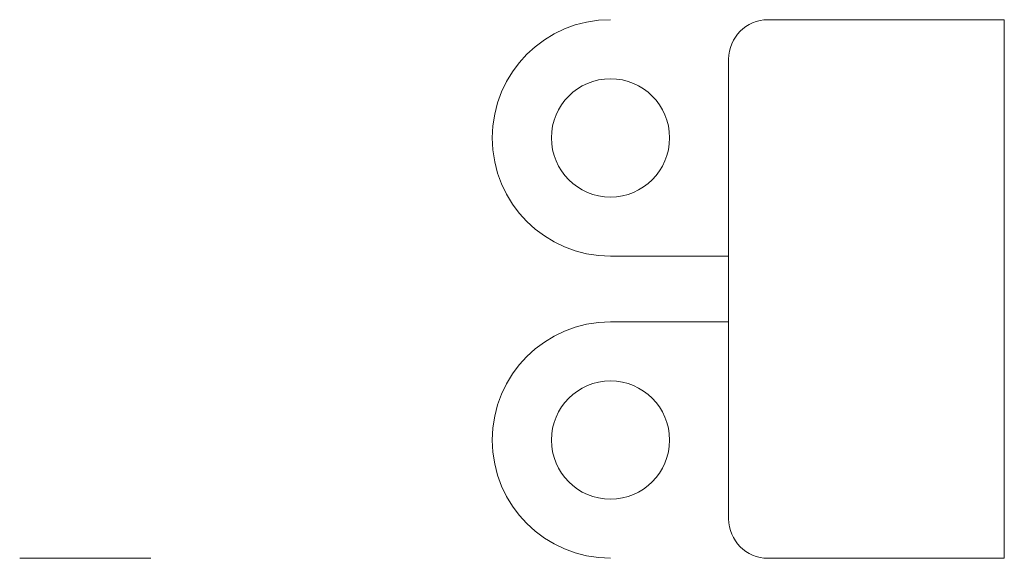
# Model space of a CAD drawing. Units: millimetres. Extents: x 2690 to 2840, y 1661 to 1743.
import ezdxf

# ---------------------------------------------------------------- set-up
doc = ezdxf.new("R2010")
doc.units = ezdxf.units.MM
doc.layers.add('M-CONS', color=8, linetype='Continuous', lineweight=18)

msp = doc.modelspace()

# ---------------------------------------------------------------- linework, layer by layer
at = {"layer": 'M-CONS'}
for p, q in [((2839.52, 1742.55, -186.73), (2803.52, 1742.55, -186.73)), ((2839.52, 1660.55, -186.73), (2839.52, 1742.55, -186.73)), ((2797.52, 1736.55, -186.73), (2797.52, 1666.55, -186.73)), ((2779.52, 1706.55, -186.73), (2797.52, 1706.55, -186.73)), ((2779.52, 1696.55, -186.73), (2797.52, 1696.55, -186.73)), ((2839.52, 1660.55, -186.73), (2803.52, 1660.55, -186.73))]:
    msp.add_line(p, q, dxfattribs=at)
at = {"layer": 'M-CONS', "extrusion": (0, -1, 0)}
for p, q in [((2689.52, 1660.55, -169.73), (2689.52, 1660.55, -186.73)), ((2709.52, 1660.55, -169.73), (2709.52, 1660.55, -186.73))]:
    msp.add_line(p, q, dxfattribs=at)
at = {"layer": 'M-CONS'}
for centre in [(2779.52, 1724.55, -186.73), (2779.52, 1678.55, -186.73)]:
    msp.add_circle(centre, 9, dxfattribs=at)
for centre, radius, start, end in [((2779.52, 1724.55, -186.73), 18, 90, 270), ((2803.52, 1736.55, -186.73), 6, 90, 180), ((2779.52, 1678.55, -186.73), 18, 90, 270), ((2803.52, 1666.55, -186.73), 6, 180, 270)]:
    msp.add_arc(centre, radius, start, end, dxfattribs=at)
at = {"layer": 'M-CONS', "extrusion": (0, -1, 0)}
msp.add_arc((2699.52, -169.73, -1660.55), 10, 0, 180, dxfattribs=at)

doc.saveas('drawing.dxf')
